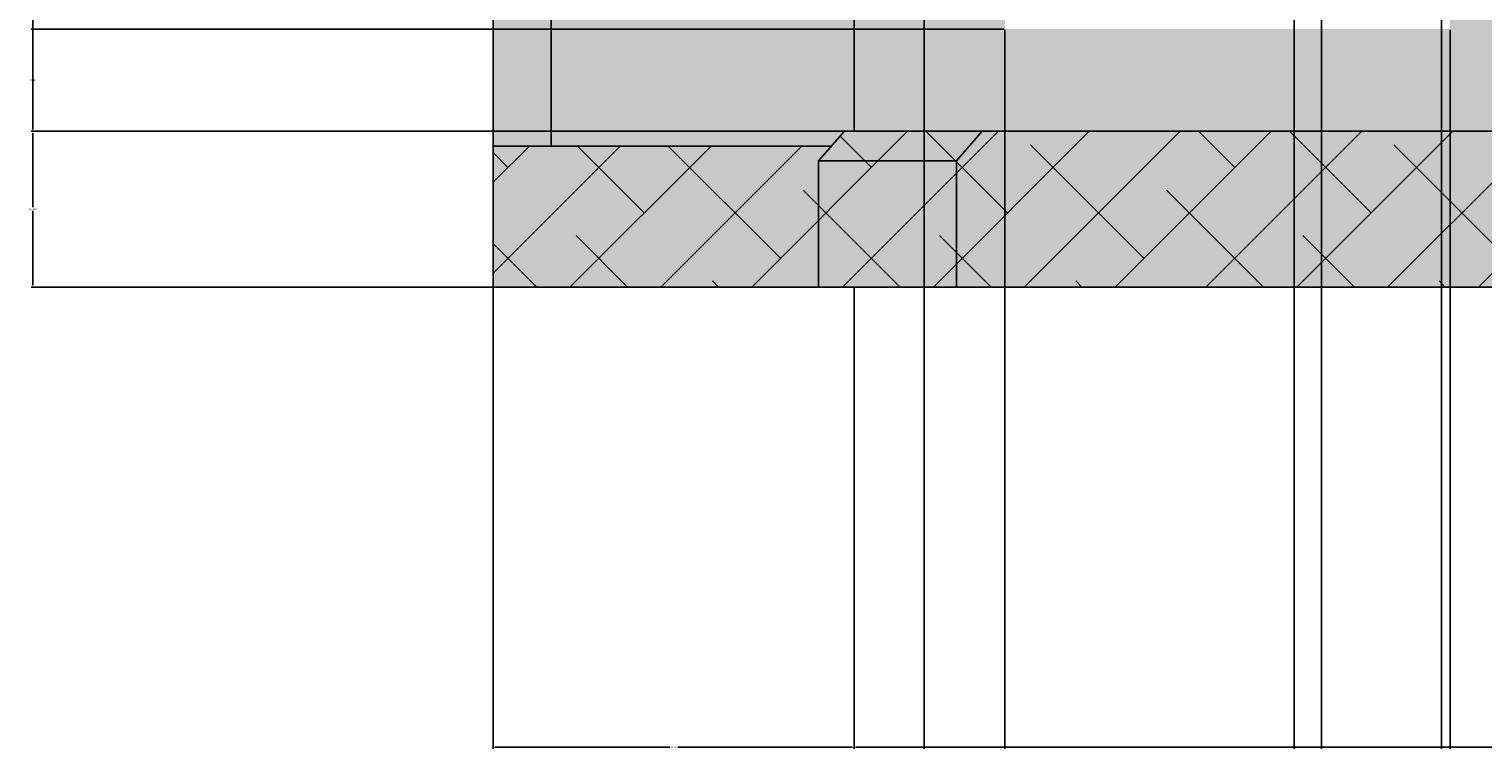
# Model space of a CAD drawing. Units: inches. Extents: x 3024 to 4744, y 1110 to 2100.
# Tile 1 of 29: x 3024 to 3168, y 1110 to 1181. Entities that reach past the tile are written whole.
import ezdxf

# ---------------------------------------------------------------- set-up
doc = ezdxf.new("R2010")
doc.units = ezdxf.units.IN
for name, color, linetype, lineweight in [('A-ANNO-DIMS', 2, 'Continuous', 18), ('A-ELEV', 7, 'Continuous', 25), ('A-ELEV-PATT', 252, 'Continuous', 13)]:
    doc.layers.add(name, color=color, linetype=linetype, lineweight=lineweight)
doc.styles.get("Standard").update_dxf_attribs({"font": 'arial.ttf'})
doc.dimstyles.get("Standard").update_dxf_attribs({"dimtxt": 0.18, "dimasz": 0.18, "dimexe": 0.18, "dimexo": 0.0625, "dimgap": 0.09, "dimtad": 0, "dimtih": 1, "dimtoh": 1, "dimdec": 1, "dimzin": 0, "dimdsep": 46, "dimlunit": 3, "dimtxsty": 'Standard', "dimcen": 0.09, "dimadec": 0, "dimazin": 0, "dimtfac": 1, "dimtdec": 1, "dimtofl": 0, "dimtmove": 0, "dimatfit": 3, "dimfxl": 1, "dimtolj": 1, "dimtzin": 0, "dimarcsym": 0})

# ---------------------------------------------------------------- blocks, each defined once
blk = doc.blocks.new('*D50')
at = {"layer": 'A-ANNO-DIMS', "color": 0, "lineweight": -2, "transparency": 16777216}
for p, q in [((3069.79, 1155.55), (3069.79, 1109.93)), ((3105.47, 1155.55), (3105.47, 1109.93)), ((3069.97, 1110.11), (3087.24, 1110.11)), ((3105.29, 1110.11), (3088.03, 1110.11))]:
    blk.add_line(p, q, dxfattribs=at)
at = {"layer": 'A-ANNO-DIMS', "color": 0, "transparency": 16777216}
for points in [[(3069.97, 1110.14), (3069.97, 1110.08), (3069.79, 1110.11)], [(3105.29, 1110.14), (3105.29, 1110.08), (3105.47, 1110.11)]]:
    blk.add_solid(points, dxfattribs=at)
at = {"layer": 'Defpoints', "color": 0, "transparency": 16777216}
for p in [(3069.79, 1155.61), (3105.47, 1155.61), (3105.47, 1110.11)]:
    blk.add_point(p, dxfattribs=at)
at = {"layer": 'A-ANNO-DIMS', "color": 0, "transparency": 16777216, "insert": (3087.63, 1110.11), "char_height": 0.18, "attachment_point": 5}
blk.add_mtext('\\A1;35.68', dxfattribs=at)
blk = doc.blocks.new('*D51')
at = {"layer": 'A-ANNO-DIMS', "color": 0, "lineweight": -2, "transparency": 16777216}
for p, q in [((3148.97, 1290.98), (3148.97, 1109.93)), ((3105.47, 1155.55), (3105.47, 1109.93)), ((3105.65, 1110.11), (3126.89, 1110.11)), ((3148.79, 1110.11), (3127.55, 1110.11))]:
    blk.add_line(p, q, dxfattribs=at)
at = {"layer": 'A-ANNO-DIMS', "color": 0, "transparency": 16777216}
for points in [[(3105.65, 1110.14), (3105.65, 1110.08), (3105.47, 1110.11)], [(3148.79, 1110.14), (3148.79, 1110.08), (3148.97, 1110.11)]]:
    blk.add_solid(points, dxfattribs=at)
at = {"layer": 'Defpoints', "color": 0, "transparency": 16777216}
for p in [(3148.97, 1291.04), (3105.47, 1155.61), (3148.97, 1110.11)]:
    blk.add_point(p, dxfattribs=at)
at = {"layer": 'A-ANNO-DIMS', "color": 0, "transparency": 16777216, "insert": (3127.22, 1110.11), "char_height": 0.18, "attachment_point": 5}
blk.add_mtext('\\A1;43.5', dxfattribs=at)
blk = doc.blocks.new('*D52')
at = {"layer": 'A-ANNO-DIMS', "color": 0, "lineweight": -2, "transparency": 16777216}
for p, q in [((3148.97, 1290.98), (3148.97, 1109.93)), ((3170.16, 1170.96), (3170.16, 1109.93)), ((3149.15, 1110.11), (3159.17, 1110.11)), ((3169.98, 1110.11), (3159.96, 1110.11))]:
    blk.add_line(p, q, dxfattribs=at)
at = {"layer": 'A-ANNO-DIMS', "color": 0, "transparency": 16777216}
for points in [[(3149.15, 1110.14), (3149.15, 1110.08), (3148.97, 1110.11)], [(3169.98, 1110.14), (3169.98, 1110.08), (3170.16, 1110.11)]]:
    blk.add_solid(points, dxfattribs=at)
at = {"layer": 'Defpoints', "color": 0, "transparency": 16777216}
for p in [(3148.97, 1291.04), (3170.16, 1171.02), (3170.16, 1110.11)]:
    blk.add_point(p, dxfattribs=at)
at = {"layer": 'A-ANNO-DIMS', "color": 0, "transparency": 16777216, "insert": (3159.57, 1110.11), "char_height": 0.18, "attachment_point": 5}
blk.add_mtext('\\A1;21.19', dxfattribs=at)
blk = doc.blocks.new('*D65')
at = {"layer": 'A-ANNO-DIMS', "color": 0, "lineweight": -2, "transparency": 16777216}
for p, q in [((3105.41, 1171.02), (3024.11, 1171.02)), ((3024.29, 1170.84), (3024.29, 1163.5)), ((3024.29, 1155.79), (3024.29, 1163.14)), ((3105.41, 1155.61), (3024.11, 1155.61))]:
    blk.add_line(p, q, dxfattribs=at)
at = {"layer": 'A-ANNO-DIMS', "color": 0, "transparency": 16777216}
for points in [[(3024.26, 1170.84), (3024.32, 1170.84), (3024.29, 1171.02)], [(3024.26, 1155.79), (3024.32, 1155.79), (3024.29, 1155.61)]]:
    blk.add_solid(points, dxfattribs=at)
at = {"layer": 'Defpoints', "color": 0, "transparency": 16777216}
for p in [(3024.29, 1171.02), (3105.47, 1171.02), (3105.47, 1155.61)]:
    blk.add_point(p, dxfattribs=at)
at = {"layer": 'A-ANNO-DIMS', "color": 0, "transparency": 16777216, "insert": (3024.29, 1163.32), "char_height": 0.18, "attachment_point": 5}
blk.add_mtext('\\A1;15.413', dxfattribs=at)
blk = doc.blocks.new('*D66')
at = {"layer": 'A-ANNO-DIMS', "color": 0, "lineweight": -2, "transparency": 16777216}
for p, q in [((3105.41, 1275.61), (3024.11, 1275.61)), ((3024.29, 1275.43), (3024.29, 1223.5)), ((3024.29, 1171.2), (3024.29, 1223.14)), ((3105.41, 1171.02), (3024.11, 1171.02))]:
    blk.add_line(p, q, dxfattribs=at)
at = {"layer": 'A-ANNO-DIMS', "color": 0, "transparency": 16777216}
for points in [[(3024.26, 1275.43), (3024.32, 1275.43), (3024.29, 1275.61)], [(3024.26, 1171.2), (3024.32, 1171.2), (3024.29, 1171.02)]]:
    blk.add_solid(points, dxfattribs=at)
at = {"layer": 'Defpoints', "color": 0, "transparency": 16777216}
for p in [(3024.29, 1275.61), (3105.47, 1275.61), (3105.47, 1171.02)]:
    blk.add_point(p, dxfattribs=at)
at = {"layer": 'A-ANNO-DIMS', "color": 0, "transparency": 16777216, "insert": (3024.29, 1223.32), "char_height": 0.18, "attachment_point": 5}
blk.add_mtext('\\A1;104.59', dxfattribs=at)
blk = doc.blocks.new('*D89')
at = {"layer": 'A-ANNO-DIMS', "color": 0, "lineweight": -2, "transparency": 16777216}
for p, q in [((3151.66, 1794.98), (3151.66, 1109.93)), ((3163.53, 1794.98), (3163.53, 1109.93)), ((3151.84, 1110.11), (3157.14, 1110.11)), ((3163.35, 1110.11), (3158.05, 1110.11))]:
    blk.add_line(p, q, dxfattribs=at)
at = {"layer": 'A-ANNO-DIMS', "color": 0, "transparency": 16777216}
for points in [[(3151.84, 1110.14), (3151.84, 1110.08), (3151.66, 1110.11)], [(3163.35, 1110.14), (3163.35, 1110.08), (3163.53, 1110.11)]]:
    blk.add_solid(points, dxfattribs=at)
at = {"layer": 'Defpoints', "color": 0, "transparency": 16777216}
for p in [(3151.66, 1795.04), (3163.53, 1795.04), (3163.53, 1110.11)]:
    blk.add_point(p, dxfattribs=at)
at = {"layer": 'A-ANNO-DIMS', "color": 0, "transparency": 16777216, "insert": (3157.59, 1110.11), "char_height": 0.18, "attachment_point": 5}
blk.add_mtext('\\A1;11.866', dxfattribs=at)
blk = doc.blocks.new('*D103')
at = {"layer": 'A-ANNO-DIMS', "color": 0, "lineweight": -2, "transparency": 16777216}
for p, q in [((3120.37, 1181.06), (3120.37, 1109.93)), ((3112.38, 1170.96), (3112.38, 1109.93)), ((3112.56, 1110.11), (3115.98, 1110.11)), ((3120.19, 1110.11), (3116.77, 1110.11))]:
    blk.add_line(p, q, dxfattribs=at)
at = {"layer": 'A-ANNO-DIMS', "color": 0, "transparency": 16777216}
for points in [[(3112.56, 1110.14), (3112.56, 1110.08), (3112.38, 1110.11)], [(3120.19, 1110.14), (3120.19, 1110.08), (3120.37, 1110.11)]]:
    blk.add_solid(points, dxfattribs=at)
at = {"layer": 'Defpoints', "color": 0, "transparency": 16777216}
for p in [(3120.37, 1181.12), (3112.38, 1171.02), (3120.37, 1110.11)]:
    blk.add_point(p, dxfattribs=at)
at = {"layer": 'A-ANNO-DIMS', "color": 0, "transparency": 16777216, "insert": (3116.38, 1110.11), "char_height": 0.18, "attachment_point": 5}
blk.add_mtext('\\A1;7.986', dxfattribs=at)
blk = doc.blocks.new('*D104')
at = {"layer": 'A-ANNO-DIMS', "color": 0, "lineweight": -2, "transparency": 16777216}
for p, q in [((3120.37, 1181.06), (3120.37, 1109.93)), ((3164.38, 1181.06), (3164.38, 1109.93)), ((3120.55, 1110.11), (3142, 1110.11)), ((3164.2, 1110.11), (3142.76, 1110.11))]:
    blk.add_line(p, q, dxfattribs=at)
at = {"layer": 'A-ANNO-DIMS', "color": 0, "transparency": 16777216}
for points in [[(3120.55, 1110.14), (3120.55, 1110.08), (3120.37, 1110.11)], [(3164.2, 1110.14), (3164.2, 1110.08), (3164.38, 1110.11)]]:
    blk.add_solid(points, dxfattribs=at)
at = {"layer": 'Defpoints', "color": 0, "transparency": 16777216}
for p in [(3120.37, 1181.12), (3164.38, 1181.12), (3164.38, 1110.11)]:
    blk.add_point(p, dxfattribs=at)
at = {"layer": 'A-ANNO-DIMS', "color": 0, "transparency": 16777216, "insert": (3142.38, 1110.11), "char_height": 0.18, "attachment_point": 5}
blk.add_mtext('\\A1;44.01', dxfattribs=at)
blk = doc.blocks.new('*D105')
at = {"layer": 'A-ANNO-DIMS', "color": 0, "lineweight": -2, "transparency": 16777216}
for p, q in [((3164.38, 1181.06), (3164.38, 1109.93)), ((3170.16, 1170.96), (3170.16, 1109.93)), ((3164.56, 1110.11), (3166.95, 1110.11)), ((3169.98, 1110.11), (3167.59, 1110.11))]:
    blk.add_line(p, q, dxfattribs=at)
at = {"layer": 'A-ANNO-DIMS', "color": 0, "transparency": 16777216}
for points in [[(3164.56, 1110.14), (3164.56, 1110.08), (3164.38, 1110.11)], [(3169.98, 1110.14), (3169.98, 1110.08), (3170.16, 1110.11)]]:
    blk.add_solid(points, dxfattribs=at)
at = {"layer": 'Defpoints', "color": 0, "transparency": 16777216}
for p in [(3164.38, 1181.12), (3170.16, 1171.02), (3170.16, 1110.11)]:
    blk.add_point(p, dxfattribs=at)
at = {"layer": 'A-ANNO-DIMS', "color": 0, "transparency": 16777216, "insert": (3167.27, 1110.11), "char_height": 0.18, "attachment_point": 5}
blk.add_mtext('\\A1;5.78', dxfattribs=at)
blk = doc.blocks.new('*D113')
at = {"layer": 'A-ANNO-DIMS', "color": 0, "lineweight": -2, "transparency": 16777216}
for p, q in [((3120.31, 1181.12), (3024.11, 1181.12)), ((3024.29, 1180.94), (3024.29, 1176.26)), ((3024.29, 1171.2), (3024.29, 1175.89)), ((3118.06, 1171.02), (3024.11, 1171.02))]:
    blk.add_line(p, q, dxfattribs=at)
at = {"layer": 'A-ANNO-DIMS', "color": 0, "transparency": 16777216}
for points in [[(3024.26, 1180.94), (3024.32, 1180.94), (3024.29, 1181.12)], [(3024.26, 1171.2), (3024.32, 1171.2), (3024.29, 1171.02)]]:
    blk.add_solid(points, dxfattribs=at)
at = {"layer": 'Defpoints', "color": 0, "transparency": 16777216}
for p in [(3024.29, 1181.12), (3120.37, 1181.12), (3118.12, 1171.02)]:
    blk.add_point(p, dxfattribs=at)
at = {"layer": 'A-ANNO-DIMS', "color": 0, "transparency": 16777216, "insert": (3024.29, 1176.07), "char_height": 0.18, "attachment_point": 5}
blk.add_mtext('\\A1;10.10', dxfattribs=at)
blk = doc.blocks.new('*D114')
at = {"layer": 'A-ANNO-DIMS', "color": 0, "lineweight": -2, "transparency": 16777216}
for p, q in [((3120.31, 1205.67), (3024.11, 1205.67)), ((3024.29, 1205.49), (3024.29, 1193.58)), ((3024.29, 1181.3), (3024.29, 1193.22)), ((3120.31, 1181.12), (3024.11, 1181.12))]:
    blk.add_line(p, q, dxfattribs=at)
at = {"layer": 'A-ANNO-DIMS', "color": 0, "transparency": 16777216}
for points in [[(3024.26, 1205.49), (3024.32, 1205.49), (3024.29, 1205.67)], [(3024.26, 1181.3), (3024.32, 1181.3), (3024.29, 1181.12)]]:
    blk.add_solid(points, dxfattribs=at)
at = {"layer": 'Defpoints', "color": 0, "transparency": 16777216}
for p in [(3024.29, 1205.67), (3120.37, 1205.67), (3120.37, 1181.12)]:
    blk.add_point(p, dxfattribs=at)
at = {"layer": 'A-ANNO-DIMS', "color": 0, "transparency": 16777216, "insert": (3024.29, 1193.4), "char_height": 0.18, "attachment_point": 5}
blk.add_mtext('\\A1;24.55', dxfattribs=at)

msp = doc.modelspace()

# ---------------------------------------------------------------- hatches: boundary and pattern name
at = {"layer": 'A-ELEV-PATT'}
h = msp.add_hatch(color=256, dxfattribs=at)
h.dxf.hatch_style = 1
h.paths.add_polyline_path([(3154.3287, 1897.4879), (3148.9694, 1897.4879), (3148.9694, 1905.6112), (3105.4722, 1905.6112), (3105.4722, 1785.6112), (3148.9694, 1785.6112), (3148.9694, 1795.0431), (3151.6604, 1795.0431), (3151.6604, 1806.8674), (3154.3287, 1806.8674)])
h.paths.add_polyline_path([(3329.7033, 1905.6112), (3292.6051, 1905.6112), (3292.6051, 1897.4879), (3287.2458, 1897.4879), (3287.2458, 1806.8674), (3288.3759, 1806.8674), (3288.3759, 1795.0431), (3292.6051, 1795.0431), (3292.6051, 1785.6112), (3329.7033, 1785.6112)])
h.paths.add_polyline_path([(3154.3287, 1771.4879), (3148.9694, 1771.4879), (3148.9694, 1779.6112), (3105.4722, 1779.6112), (3105.4722, 1659.6112), (3148.9694, 1659.6112), (3148.9694, 1669.0431), (3151.6604, 1669.0431), (3151.6604, 1680.8674), (3154.3287, 1680.8674)])
h.paths.add_polyline_path([(3329.7033, 1779.6112), (3292.6051, 1779.6112), (3292.6051, 1771.4879), (3287.2458, 1771.4879), (3287.2458, 1680.8674), (3288.3759, 1680.8674), (3288.3759, 1669.0431), (3292.6051, 1669.0431), (3292.6051, 1659.6112), (3329.7033, 1659.6112)])
h.paths.add_polyline_path([(3154.3287, 1645.4879), (3148.9694, 1645.4879), (3148.9694, 1653.6112), (3105.4722, 1653.6112), (3105.4722, 1533.6112), (3148.9694, 1533.6112), (3148.9694, 1543.0431), (3151.6604, 1543.0431), (3151.6604, 1554.8674), (3154.3287, 1554.8674)])
h.paths.add_polyline_path([(3329.7033, 1653.6112), (3292.6051, 1653.6112), (3292.6051, 1645.4879), (3287.2458, 1645.4879), (3287.2458, 1554.8674), (3288.3759, 1554.8674), (3288.3759, 1543.0431), (3292.6051, 1543.0431), (3292.6051, 1533.6112), (3329.7033, 1533.6112)])
h.paths.add_polyline_path([(3329.7033, 1527.6112), (3292.6051, 1527.6112), (3292.6051, 1519.4879), (3287.2458, 1519.4879), (3287.2458, 1428.8674), (3288.3759, 1428.8674), (3288.3759, 1417.0431), (3292.6051, 1417.0431), (3292.6051, 1407.6112), (3329.7033, 1407.6112)])
h.paths.add_polyline_path([(3329.7033, 1401.6112), (3292.6051, 1401.6112), (3292.6051, 1393.4879), (3287.2458, 1393.4879), (3287.2458, 1302.8674), (3288.3759, 1302.8674), (3288.3759, 1291.0431), (3292.6051, 1291.0431), (3292.6051, 1281.6112), (3329.7033, 1281.6112)])
h.paths.add_polyline_path([(3154.3287, 1393.4879), (3148.9694, 1393.4879), (3148.9694, 1401.6112), (3105.4722, 1401.6112), (3105.4722, 1281.6112), (3148.9694, 1281.6112), (3148.9694, 1291.0431), (3151.6604, 1291.0431), (3151.6604, 1302.8674), (3154.3287, 1302.8674)])
h.paths.add_polyline_path([(3154.3287, 1519.4879), (3148.9694, 1519.4879), (3148.9694, 1527.6112), (3105.4722, 1527.6112), (3105.4722, 1407.6112), (3148.9694, 1407.6112), (3148.9694, 1417.0431), (3151.6604, 1417.0431), (3151.6604, 1428.8674), (3154.3287, 1428.8674)])
h.paths.add_polyline_path([(3515.7606, 1897.4879), (3510.4013, 1897.4879), (3510.4013, 1905.6112), (3481.2411, 1905.6112), (3481.2411, 1785.6112), (3510.4013, 1785.6112), (3510.4013, 1795.0431), (3513.0923, 1795.0431), (3513.0923, 1806.8674), (3515.7606, 1806.8674)])
h.paths.add_polyline_path([(3688.5588, 1905.6112), (3654.037, 1905.6112), (3654.037, 1897.4879), (3648.6777, 1897.4879), (3648.6777, 1806.8674), (3649.8078, 1806.8674), (3649.8078, 1795.0431), (3654.037, 1795.0431), (3654.037, 1785.6112), (3688.5588, 1785.6112)])
h.paths.add_polyline_path([(3515.7606, 1771.4879), (3510.4013, 1771.4879), (3510.4013, 1779.6112), (3481.2411, 1779.6112), (3481.2411, 1659.6112), (3510.4013, 1659.6112), (3510.4013, 1669.0431), (3513.0923, 1669.0431), (3513.0923, 1680.8674), (3515.7606, 1680.8674)])
h.paths.add_polyline_path([(3688.5588, 1779.6112), (3654.037, 1779.6112), (3654.037, 1771.4879), (3648.6777, 1771.4879), (3648.6777, 1680.8674), (3649.8078, 1680.8674), (3649.8078, 1669.0431), (3654.037, 1669.0431), (3654.037, 1659.6112), (3688.5588, 1659.6112)])
h.paths.add_polyline_path([(3515.7606, 1645.4879), (3510.4013, 1645.4879), (3510.4013, 1653.6112), (3481.2411, 1653.6112), (3481.2411, 1533.6112), (3510.4013, 1533.6112), (3510.4013, 1543.0431), (3513.0923, 1543.0431), (3513.0923, 1554.8674), (3515.7606, 1554.8674)])
h.paths.add_polyline_path([(3688.5588, 1653.6112), (3654.037, 1653.6112), (3654.037, 1645.4879), (3648.6777, 1645.4879), (3648.6777, 1554.8674), (3649.8078, 1554.8674), (3649.8078, 1543.0431), (3654.037, 1543.0431), (3654.037, 1533.6112), (3688.5588, 1533.6112)])
h.paths.add_polyline_path([(3515.7606, 1519.4879), (3510.4013, 1519.4879), (3510.4013, 1527.6112), (3481.2411, 1527.6112), (3481.2411, 1407.6112), (3510.4013, 1407.6112), (3510.4013, 1417.0431), (3513.0923, 1417.0431), (3513.0923, 1428.8674), (3515.7606, 1428.8674)])
h.paths.add_polyline_path([(3688.5588, 1527.6112), (3654.037, 1527.6112), (3654.037, 1519.4879), (3648.6777, 1519.4879), (3648.6777, 1428.8674), (3649.8078, 1428.8674), (3649.8078, 1417.0431), (3654.037, 1417.0431), (3654.037, 1407.6112), (3688.5588, 1407.6112)])
h.paths.add_polyline_path([(3515.7606, 1393.4879), (3510.4013, 1393.4879), (3510.4013, 1401.6112), (3481.2411, 1401.6112), (3481.2411, 1281.6112), (3510.4013, 1281.6112), (3510.4013, 1291.0431), (3513.0923, 1291.0431), (3513.0923, 1302.8674), (3515.7606, 1302.8674)])
h.paths.add_polyline_path([(3688.5588, 1401.6112), (3654.037, 1401.6112), (3654.037, 1393.4879), (3648.6777, 1393.4879), (3648.6777, 1302.8674), (3649.8078, 1302.8674), (3649.8078, 1291.0431), (3654.037, 1291.0431), (3654.037, 1281.6112), (3688.5588, 1281.6112)])
h.paths.add_polyline_path([(3515.7606, 1267.4879), (3510.4013, 1267.4879), (3510.4013, 1275.6112), (3481.2411, 1275.6112), (3481.2411, 1155.6112), (3510.4013, 1155.6112), (3510.4013, 1165.0431), (3513.0923, 1165.0431), (3513.0923, 1176.8674), (3515.7606, 1176.8674)])
h.paths.add_polyline_path([(3688.5588, 1275.6112), (3654.037, 1275.6112), (3654.037, 1267.4879), (3648.6777, 1267.4879), (3648.6777, 1176.8674), (3649.8078, 1176.8674), (3649.8078, 1165.0431), (3654.037, 1165.0431), (3654.037, 1155.6112), (3688.5588, 1155.6112)])
h.paths.add_polyline_path([(3112.3838, 1275.6112), (3105.4722, 1275.6112), (3105.4722, 1171.0239), (3112.3838, 1171.0239)])
h = msp.add_hatch(color=256, dxfattribs=at)
h.dxf.hatch_style = 1
h.paths.add_polyline_path([(3329.7033, 1275.6112), (3274.3877, 1275.6112), (3274.3877, 1171.0239), (3329.7033, 1171.0239)])
h.paths.add_polyline_path([(3323.3693, 1246.0161), (3279.3584, 1246.0161), (3279.3584, 1270.5642), (3323.3693, 1270.5642)], flags=16)
h.paths.add_polyline_path([(3323.3693, 1238.118), (3323.3693, 1213.5699), (3279.3584, 1213.5699), (3279.3584, 1238.118)], flags=16)
h.paths.add_polyline_path([(3323.3693, 1205.6718), (3323.3693, 1181.1236), (3279.3584, 1181.1236), (3279.3584, 1205.6718)], flags=16)
h.paths.add_polyline_path([(3170.1608, 1275.6112), (3112.3838, 1275.6112), (3112.3838, 1171.0239), (3118.1176, 1171.0239), (3170.1608, 1171.0239)])
h.paths.add_polyline_path([(3120.3696, 1246.0161), (3120.3696, 1270.5642), (3164.3806, 1270.5642), (3164.3806, 1246.0161)], flags=16)
h.paths.add_polyline_path([(3120.3696, 1238.118), (3164.3806, 1238.118), (3164.3806, 1213.5699), (3120.3696, 1213.5699)], flags=16)
h.paths.add_polyline_path([(3120.3696, 1205.6718), (3164.3806, 1205.6718), (3164.3806, 1181.1236), (3120.3696, 1181.1236)], flags=16)
h = msp.add_hatch(color=256, dxfattribs=at)
h.dxf.hatch_style = 1
h.paths.add_polyline_path([(3329.7033, 1171.0239), (3256.7794, 1171.0239, -0.21182003), (3255.8005, 1171.0239), (3249.6327, 1171.0239, -0.21182003), (3248.6539, 1171.0239), (3195.8947, 1171.0239, -0.21182003), (3194.9159, 1171.0239), (3188.7481, 1171.0239, -0.21182003), (3187.7692, 1171.0239), (3118.1176, 1171.0239), (3115.5754, 1168.0828), (3115.5754, 1155.6112), (3329.7033, 1155.6112)])
h.paths.add_polyline_path([(3101.9647, 1168.0828), (3103.2358, 1169.5534), (3069.7937, 1169.5534), (3069.7937, 1155.6112), (3101.9647, 1155.6112)])
h.paths.add_polyline_path([(3115.5754, 1168.0828), (3101.9647, 1168.0828), (3101.9647, 1155.6112), (3105.4722, 1155.6112), (3115.5754, 1155.6112)])
h.paths.add_polyline_path([(3118.1176, 1171.0239), (3104.5069, 1171.0239), (3101.9647, 1168.0828), (3115.5754, 1168.0828)])
h.paths.add_polyline_path([(3105.4722, 1265.3254), (3075.5369, 1241.4341), (3075.5369, 1169.5534), (3103.2358, 1169.5534), (3104.5069, 1171.0239), (3105.4722, 1171.0239)])
h.paths.add_polyline_path([(3105.4722, 1265.3254), (3105.4722, 1269.9091), (3069.7937, 1241.4341), (3075.5369, 1241.4341)])
h.paths.add_polyline_path([(3075.5369, 1241.4341), (3069.7937, 1241.4341), (3069.7937, 1169.5534), (3075.5369, 1169.5534)])
h.paths.add_polyline_path([(3735.4075, 1241.4341), (3705.4722, 1265.3254), (3705.4722, 1169.5534), (3735.4075, 1169.5534)])
h.paths.add_polyline_path([(3705.4722, 1269.9091), (3705.4722, 1265.3254), (3735.4075, 1241.4341), (3741.1507, 1241.4341)])
h.paths.add_polyline_path([(3741.1507, 1241.4341), (3735.4075, 1241.4341), (3735.4075, 1169.5534), (3741.1507, 1169.5534)])
h.paths.add_polyline_path([(3741.1507, 1169.5534), (3735.4075, 1169.5534), (3705.4722, 1169.5534), (3705.4722, 1155.6112), (3741.1507, 1155.6112)])
h = msp.add_hatch(dxfattribs=at)
h.set_pattern_fill('AR-B816', color=256, scale=0.01)
h.paths.add_polyline_path([(3105.4722, 1265.3254), (3075.5369, 1241.4341), (3075.5369, 1169.5534), (3103.2358, 1169.5534), (3104.5069, 1171.0239), (3105.4722, 1171.0239)])
h.paths.add_polyline_path([(3105.4722, 1265.3254), (3105.4722, 1269.9091), (3069.7937, 1241.4341), (3075.5369, 1241.4341)])
h.paths.add_polyline_path([(3075.5369, 1241.4341), (3069.7937, 1241.4341), (3069.7937, 1169.5534), (3075.5369, 1169.5534)])
h.paths.add_polyline_path([(3735.4075, 1241.4341), (3705.4722, 1265.3254), (3705.4722, 1169.5534), (3735.4075, 1169.5534)])
h.paths.add_polyline_path([(3705.4722, 1269.9091), (3705.4722, 1265.3254), (3735.4075, 1241.4341), (3741.1507, 1241.4341)])
h.paths.add_polyline_path([(3741.1507, 1241.4341), (3735.4075, 1241.4341), (3735.4075, 1169.5534), (3741.1507, 1169.5534)])
h = msp.add_hatch(dxfattribs=at)
h.set_pattern_fill('ANSI38', color=256, scale=2)
h.paths.add_polyline_path([(3101.9647, 1168.0828), (3103.2358, 1169.5534), (3069.7937, 1169.5534), (3069.7937, 1155.6112), (3101.9647, 1155.6112)])
h.paths.add_polyline_path([(3115.5754, 1168.0828), (3101.9647, 1168.0828), (3101.9647, 1155.6112), (3105.4722, 1155.6112), (3115.5754, 1155.6112)])
h.paths.add_polyline_path([(3118.1176, 1171.0239), (3104.5069, 1171.0239), (3101.9647, 1168.0828), (3115.5754, 1168.0828)])
h.paths.add_polyline_path([(3329.7033, 1171.0239), (3256.7794, 1171.0239, -0.21182003), (3255.8005, 1171.0239), (3249.6327, 1171.0239, -0.21182003), (3248.6539, 1171.0239), (3195.8947, 1171.0239, -0.21182003), (3194.9159, 1171.0239), (3188.7481, 1171.0239, -0.21182003), (3187.7692, 1171.0239), (3118.1176, 1171.0239), (3115.5754, 1168.0828), (3115.5754, 1155.6112), (3329.7033, 1155.6112)])
h.paths.add_polyline_path([(3741.1507, 1169.5534), (3735.4075, 1169.5534), (3705.4722, 1169.5534), (3705.4722, 1155.6112), (3741.1507, 1155.6112)])

# ---------------------------------------------------------------- linework, layer by layer
at = {"layer": 'A-ELEV'}
for p, q in [((3105.4722, 1171.0239), (3105.4722, 1905.6112)), ((3105.4722, 1171.0239), (3105.4722, 1905.6112)), ((3101.9647, 1168.0828), (3104.5069, 1171.0239)), ((3101.9647, 1168.0828), (3104.5069, 1171.0239)), ((3104.5069, 1171.0239), (3118.1176, 1171.0239)), ((3104.5069, 1171.0239), (3118.1176, 1171.0239)), ((3115.5754, 1168.0828), (3118.1176, 1171.0239)), ((3115.5754, 1168.0828), (3118.1176, 1171.0239)), ((3118.1176, 1171.0239), (3329.7033, 1171.0239)), ((3118.1176, 1171.0239), (3329.7033, 1171.0239)), ((3069.7937, 1155.6112), (3069.7937, 1169.5534)), ((3103.2358, 1169.5534), (3069.7937, 1169.5534)), ((3069.7937, 1155.6112), (3069.7937, 1169.5534)), ((3103.2358, 1169.5534), (3069.7937, 1169.5534)), ((3101.9647, 1168.0828), (3115.5754, 1168.0828)), ((3101.9647, 1168.0828), (3115.5754, 1168.0828)), ((3105.4722, 1155.6112), (3069.7937, 1155.6112)), ((3105.4722, 1155.6112), (3069.7937, 1155.6112)), ((3105.4722, 1155.6112), (3705.4722, 1155.6112)), ((3105.4722, 1155.6112), (3705.4722, 1155.6112))]:
    msp.add_line(p, q, dxfattribs=at)
for points in [[(3105.4722, 1275.6112), (3112.3838, 1275.6112), (3112.3838, 1171.0239)], [(3105.4722, 1275.6112), (3112.3838, 1275.6112), (3112.3838, 1171.0239)], [(3115.5754, 1155.6112), (3115.5754, 1168.0828), (3101.9647, 1168.0828), (3101.9647, 1155.6112)], [(3115.5754, 1155.6112), (3115.5754, 1168.0828), (3101.9647, 1168.0828), (3101.9647, 1155.6112)]]:
    msp.add_lwpolyline(points, dxfattribs=at)
msp.add_lwpolyline([(3069.7937, 1169.5534), (3075.5369, 1169.5534), (3075.5369, 1241.4341), (3069.7937, 1241.4341)], close=True, dxfattribs=at)
msp.add_lwpolyline([(3069.7937, 1169.5534), (3075.5369, 1169.5534), (3075.5369, 1241.4341), (3069.7937, 1241.4341)], close=True, dxfattribs=at)

# ---------------------------------------------------------------- dimensions: what is measured, and where the dimension line sits
at = {"layer": 'A-ANNO-DIMS'}
for base, p1, p2, override, picture, middle in [((3163.526875, 1110.111173), (3151.660378, 1795.043127), (3163.526875, 1795.043127), {"dimdec": 3, "dimlfac": 1, "dimrnd": 0, "dimzin": 0, "dimdsep": 46, "dimlunit": 2}, '*D89', (3157.593627, 1110.111173)), ((3148.9694, 1110.1112), (3105.4722, 1155.6112), (3148.9694, 1291.0431), {"dimdec": 1, "dimlfac": 1, "dimrnd": 0, "dimzin": 0, "dimdsep": 46, "dimlunit": 2}, '*D51', (3127.2208, 1110.1112)), ((3170.1608, 1110.1112), (3148.9694, 1291.0431), (3170.1608, 1171.0239), {"dimdec": 2, "dimlfac": 1, "dimrnd": 0, "dimzin": 0, "dimdsep": 46, "dimlunit": 2}, '*D52', (3159.5651, 1110.1112)), ((3120.3696, 1110.1112), (3112.3838, 1171.0239), (3120.3696, 1181.1236), {"dimdec": 3, "dimlfac": 1, "dimrnd": 0, "dimzin": 0, "dimdsep": 46, "dimlunit": 2}, '*D103', (3116.3767, 1110.1112)), ((3164.3806, 1110.1112), (3120.3696, 1181.1236), (3164.3806, 1181.1236), {"dimdec": 2, "dimlfac": 1, "dimrnd": 0, "dimzin": 0, "dimdsep": 46, "dimlunit": 2}, '*D104', (3142.3751, 1110.1112)), ((3170.1608, 1110.1112), (3164.3806, 1181.1236), (3170.1608, 1171.0239), {"dimdec": 2, "dimlfac": 1, "dimrnd": 0, "dimzin": 0, "dimdsep": 46, "dimlunit": 2}, '*D105', (3167.2707, 1110.1112)), ((3105.4722, 1110.1112), (3069.7937, 1155.6112), (3105.4722, 1155.6112), {"dimdec": 2, "dimlfac": 1, "dimrnd": 0, "dimzin": 0, "dimdsep": 46, "dimlunit": 2}, '*D50', (3087.6329, 1110.1112))]:
    dim = msp.add_linear_dim(base=base, p1=p1, p2=p2, dimstyle='Standard', override=override, dxfattribs=at)
    dim.commit()
    dim.dimension.update_dxf_attribs({"geometry": picture, "text_midpoint": middle})
for base, p1, p2, override, picture, middle in [((3024.2937, 1275.6112), (3105.4722, 1171.0239), (3105.4722, 1275.6112), {"dimdec": 2, "dimlfac": 1, "dimrnd": 0, "dimzin": 0, "dimdsep": 46, "dimlunit": 2}, '*D66', (3024.2937, 1223.3176)), ((3024.2937, 1205.6718), (3120.3696, 1181.1236), (3120.3696, 1205.6718), {"dimdec": 2, "dimlfac": 1, "dimrnd": 0, "dimzin": 0, "dimdsep": 46, "dimlunit": 2}, '*D114', (3024.2937, 1193.3977)), ((3024.2937, 1181.1236), (3118.1176, 1171.0239), (3120.3696, 1181.1236), {"dimdec": 2, "dimlfac": 1, "dimrnd": 0, "dimzin": 0, "dimdsep": 46, "dimlunit": 2}, '*D113', (3024.2937, 1176.0738)), ((3024.2937, 1171.0239), (3105.4722, 1155.6112), (3105.4722, 1171.0239), {"dimdec": 3, "dimlfac": 1, "dimrnd": 0, "dimzin": 0, "dimdsep": 46, "dimlunit": 2}, '*D65', (3024.2937, 1163.3176))]:
    dim = msp.add_linear_dim(base=base, p1=p1, p2=p2, angle=90, dimstyle='Standard', override=override, dxfattribs=at)
    dim.commit()
    dim.dimension.update_dxf_attribs({"geometry": picture, "text_midpoint": middle})

doc.saveas('drawing.dxf')
